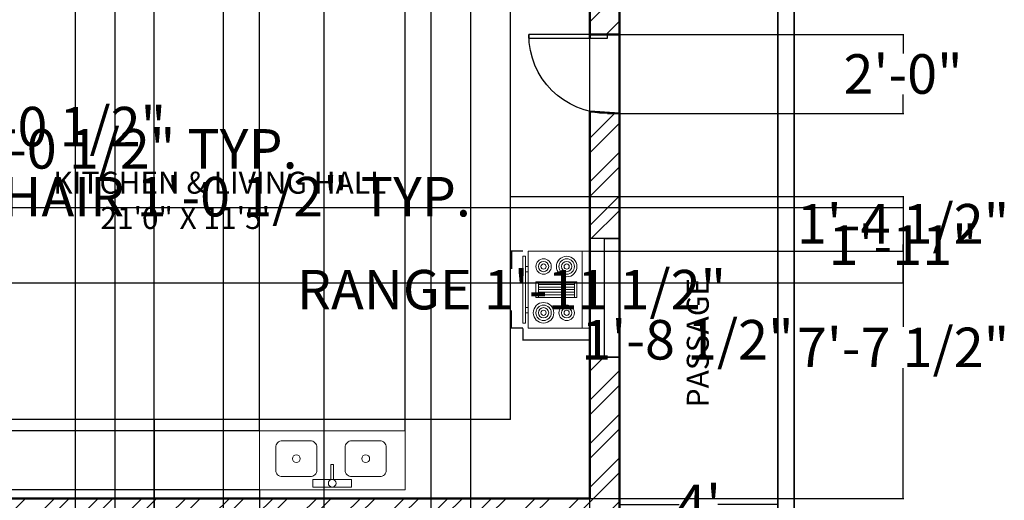
# Model space of a CAD drawing. Units: inches. Extents: x -40 to 578, y -482 to 237.
# Tile 6 of 7: x 249 to 548, y -129 to 17. Entities that reach past the tile are written whole.
import ezdxf

# ---------------------------------------------------------------- set-up
doc = ezdxf.new("R2010")
doc.units = ezdxf.units.IN
doc.header["$MEASUREMENT"] = 0
for name, color, linetype, lineweight in [('A-ANNO-DIMS', 2, 'Continuous', 18), ('A-AREA-IDEN', 240, 'Continuous', 25), ('A-EQPM', 4, 'Continuous', 18), ('A-FLOR-CASE', 4, 'Continuous', 25), ('A-FLOR-FIXT', 4, 'Continuous', 18), ('A-WALL-PATT', 252, 'Continuous', 13), ('C-PROP', 3, 'Continuous', 35), ('DOORS', 2, 'Continuous', 25), ('WALLS', 3, 'Continuous', 50), ('WINDOWS', 241, 'Continuous', 25)]:
    doc.layers.add(name, color=color, linetype=linetype, lineweight=lineweight)
doc.styles.get("Standard").update_dxf_attribs({"font": 'arial.ttf'})
doc.dimstyles.get("Standard").update_dxf_attribs({"dimtxt": 12, "dimasz": 0.18, "dimexe": 0.18, "dimexo": 0.0625, "dimgap": 0.09, "dimtad": 0, "dimtih": 1, "dimtoh": 1, "dimdec": 0, "dimzin": 0, "dimdsep": 46, "dimlunit": 3, "dimtxsty": 'Standard', "dimcen": 0.09, "dimadec": 0, "dimazin": 0, "dimtfac": 1, "dimtdec": 0, "dimtofl": 0, "dimtmove": 0, "dimatfit": 3, "dimfxl": 1, "dimtolj": 1, "dimtzin": 0, "dimarcsym": 0})

# ---------------------------------------------------------------- blocks, each defined once
blk = doc.blocks.new('Range-Oven - 30 in top')
for p, q in [((0, -3), (30, -3)), ((12, -6), (18, -6)), ((13, -20), (13, -6)), ((14, -6), (14, -20)), ((15, -20), (15, -6)), ((16, -6), (16, -20)), ((17, -20), (17, -6)), ((18, -20), (12, -20)), ((6, -24), (6, -25)), ((8, -25), (8, -24)), ((22, -25), (22, -24)), ((24, -24), (24, -25))]:
    blk.add_line(p, q)
for points in [[(0, -24), (0, 0), (30, 0), (30, -24)], [(12, -21), (12, -5), (18, -5), (18, -21)], [(2, -26), (2, -25), (28, -25), (28, -26)]]:
    blk.add_lwpolyline(points, close=True)
for centre, radius in [((6, -9), 4), ((6, -9), 3), ((6, -9), 2), ((24, -9), 3), ((24, -9), 2), ((6, -9), 1), ((24, -9), 1), ((6, -18), 3), ((24, -18), 4), ((24, -18), 3), ((6, -18), 2), ((6, -18), 1), ((24, -18), 2), ((24, -18), 1)]:
    blk.add_circle(centre, radius)
blk = doc.blocks.new('*U10')
for p, q in [((0, 0), (0, -6)), ((40, 0), (40, -6))]:
    blk.add_line(p, q)
blk.add_lwpolyline([(0, 0), (0, 40), (1.75, 40), (1.75, 0)], close=True)
blk.add_arc((0, 0), 40, 0, 90)
blk = doc.blocks.new('*D19')
at = {"layer": 'A-ANNO-DIMS', "color": 0, "lineweight": -2, "transparency": 16777216}
for p, q in [((430.74, -125.2), (430.74, -130.58)), ((478.74, -125.2), (478.74, -130.58)), ((430.92, -130.4), (448.89, -130.4)), ((478.56, -130.4), (460.59, -130.4))]:
    blk.add_line(p, q, dxfattribs=at)
at = {"layer": 'A-ANNO-DIMS', "color": 0, "transparency": 16777216}
for points in [[(430.92, -130.37), (430.92, -130.43), (430.74, -130.4)], [(478.56, -130.37), (478.56, -130.43), (478.74, -130.4)]]:
    blk.add_solid(points, dxfattribs=at)
at = {"layer": 'Defpoints', "color": 0, "transparency": 16777216}
for p in [(430.74, -125.13), (478.74, -125.13), (478.74, -130.4)]:
    blk.add_point(p, dxfattribs=at)
at = {"layer": 'A-ANNO-DIMS', "color": 0, "transparency": 16777216, "insert": (454.74, -130.4), "char_height": 12, "attachment_point": 5}
blk.add_mtext("\\A1;4'", dxfattribs=at)
blk = doc.blocks.new('WIN-36IN')
for p, q in [((9, 36), (0, 36)), ((4.5, 0), (4.5, 36)), ((4.5, 36), (9, 36)), ((9, 0), (0, 0)), ((4.5, 0), (9, 0))]:
    blk.add_line(p, q)
blk = doc.blocks.new('*D30')
at = {"layer": 'A-ANNO-DIMS', "color": 0, "lineweight": -2, "transparency": 16777216}
for p, q in [((217.52, -35.11), (217.52, -37.13)), ((230.16, -35.11), (230.16, -37.13)), ((217.7, -36.95), (229.98, -36.95)), ((230.16, -36.95), (230.34, -36.95))]:
    blk.add_line(p, q, dxfattribs=at)
at = {"layer": 'A-ANNO-DIMS', "color": 0, "transparency": 16777216}
for points in [[(217.7, -36.92), (217.7, -36.98), (217.52, -36.95)], [(229.98, -36.92), (229.98, -36.98), (230.16, -36.95)]]:
    blk.add_solid(points, dxfattribs=at)
at = {"layer": 'Defpoints', "color": 0, "transparency": 16777216}
for p in [(217.52, -35.05), (230.16, -35.05), (230.16, -36.95)]:
    blk.add_point(p, dxfattribs=at)
at = {"layer": 'A-ANNO-DIMS', "color": 0, "transparency": 16777216, "insert": (309.32, -36.95), "char_height": 12, "attachment_point": 5}
blk.add_mtext('\\A1;CHAIR 1\'-0 1/2" TYP.', dxfattribs=at)
blk = doc.blocks.new('*D31')
at = {"layer": 'A-ANNO-DIMS', "color": 0, "lineweight": -2, "transparency": 16777216}
for p, q in [((230.22, -22.61), (232.23, -22.61)), ((232.05, -22.61), (232.05, -22.43)), ((232.05, -22.43), (232.23, -22.43)), ((232.05, -34.87), (232.05, -22.79)), ((230.22, -35.05), (232.23, -35.05))]:
    blk.add_line(p, q, dxfattribs=at)
at = {"layer": 'A-ANNO-DIMS', "color": 0, "transparency": 16777216}
for points in [[(232.02, -22.79), (232.08, -22.79), (232.05, -22.61)], [(232.02, -34.87), (232.08, -34.87), (232.05, -35.05)]]:
    blk.add_solid(points, dxfattribs=at)
at = {"layer": 'Defpoints', "color": 0, "transparency": 16777216}
for p in [(230.16, -22.61), (232.05, -22.61), (230.16, -35.05)]:
    blk.add_point(p, dxfattribs=at)
at = {"layer": 'A-ANNO-DIMS', "color": 0, "transparency": 16777216, "insert": (282.31, -22.43), "char_height": 12, "attachment_point": 5}
blk.add_mtext('\\A1;1\'-0 1/2" TYP.', dxfattribs=at)
blk = doc.blocks.new('*D40')
at = {"layer": 'A-ANNO-DIMS', "color": 0, "lineweight": -2, "transparency": 16777216}
for p, q in [((401.4, -53.48), (397.77, -53.48)), ((397.95, -53.66), (397.95, -58.88)), ((397.95, -76.7), (397.95, -71.47)), ((401.4, -76.88), (397.77, -76.88))]:
    blk.add_line(p, q, dxfattribs=at)
at = {"layer": 'A-ANNO-DIMS', "color": 0, "transparency": 16777216}
for points in [[(397.92, -53.66), (397.98, -53.66), (397.95, -53.48)], [(397.92, -76.7), (397.98, -76.7), (397.95, -76.88)]]:
    blk.add_solid(points, dxfattribs=at)
at = {"layer": 'Defpoints', "color": 0, "transparency": 16777216}
for p in [(401.46, -53.48), (397.95, -76.88), (401.46, -76.88)]:
    blk.add_point(p, dxfattribs=at)
at = {"layer": 'A-ANNO-DIMS', "color": 0, "transparency": 16777216, "insert": (397.95, -65.18), "char_height": 12, "attachment_point": 5}
blk.add_mtext('\\A1;RANGE 1\'-11 1/2"', dxfattribs=at)
blk = doc.blocks.new('*D41')
at = {"layer": 'A-ANNO-DIMS', "color": 0, "lineweight": -2, "transparency": 16777216}
for p, q in [((401.46, -76.94), (401.46, -80.57)), ((421.74, -76.94), (421.74, -80.57)), ((401.64, -80.39), (421.56, -80.39)), ((421.74, -80.39), (421.92, -80.39))]:
    blk.add_line(p, q, dxfattribs=at)
at = {"layer": 'A-ANNO-DIMS', "color": 0, "transparency": 16777216}
for points in [[(401.64, -80.36), (401.64, -80.42), (401.46, -80.39)], [(421.56, -80.36), (421.56, -80.42), (421.74, -80.39)]]:
    blk.add_solid(points, dxfattribs=at)
at = {"layer": 'Defpoints', "color": 0, "transparency": 16777216}
for p in [(401.46, -76.88), (421.74, -76.88), (421.74, -80.39)]:
    blk.add_point(p, dxfattribs=at)
at = {"layer": 'A-ANNO-DIMS', "color": 0, "transparency": 16777216, "insert": (451.37, -80.39), "char_height": 12, "attachment_point": 5}
blk.add_mtext('\\A1;1\'-8 1/2"', dxfattribs=at)
blk = doc.blocks.new('*D49')
at = {"layer": 'A-ANNO-DIMS', "color": 0, "lineweight": -2, "transparency": 16777216}
for p, q in [((385.66, -377.49), (385.66, 219.12)), ((385.84, 218.94), (387.66, 218.94)), ((421.56, 218.94), (419.73, 218.94)), ((421.74, -377.49), (421.74, 219.12))]:
    blk.add_line(p, q, dxfattribs=at)
at = {"layer": 'A-ANNO-DIMS', "color": 0, "transparency": 16777216}
for points in [[(385.84, 218.97), (385.84, 218.91), (385.66, 218.94)], [(421.56, 218.97), (421.56, 218.91), (421.74, 218.94)]]:
    blk.add_solid(points, dxfattribs=at)
at = {"layer": 'Defpoints', "color": 0, "transparency": 16777216}
for p in [(421.74, 218.94), (385.66, -377.55), (421.74, -377.55)]:
    blk.add_point(p, dxfattribs=at)
at = {"layer": 'A-ANNO-DIMS', "color": 0, "transparency": 16777216, "insert": (403.7, 218.94), "char_height": 12, "attachment_point": 5}
blk.add_mtext('\\A1;3\'-0"', dxfattribs=at)
blk = doc.blocks.new('*D50')
at = {"layer": 'A-ANNO-DIMS', "color": 0, "lineweight": -2, "transparency": 16777216}
for p, q in [((265.66, -330.99), (265.66, 219.12)), ((265.84, 218.94), (277.48, 218.94)), ((277.66, -330.99), (277.66, 219.12)), ((277.66, 218.94), (277.84, 218.94))]:
    blk.add_line(p, q, dxfattribs=at)
at = {"layer": 'A-ANNO-DIMS', "color": 0, "transparency": 16777216}
for points in [[(265.84, 218.97), (265.84, 218.91), (265.66, 218.94)], [(277.48, 218.97), (277.48, 218.91), (277.66, 218.94)]]:
    blk.add_solid(points, dxfattribs=at)
at = {"layer": 'Defpoints', "color": 0, "transparency": 16777216}
for p in [(277.66, 218.94), (265.66, -331.05), (277.66, -331.05)]:
    blk.add_point(p, dxfattribs=at)
at = {"layer": 'A-ANNO-DIMS', "color": 0, "transparency": 16777216, "insert": (293.31, 218.94), "char_height": 12, "attachment_point": 5}
blk.add_mtext('\\A1;1\'-0"', dxfattribs=at)
blk = doc.blocks.new('*D52')
at = {"layer": 'A-ANNO-DIMS', "color": 0, "lineweight": -2, "transparency": 16777216}
for p, q in [((234.57, -377.49), (234.57, 219.12)), ((234.75, 218.94), (265.48, 218.94)), ((265.66, -377.49), (265.66, 219.12)), ((265.66, 218.94), (265.84, 218.94))]:
    blk.add_line(p, q, dxfattribs=at)
at = {"layer": 'A-ANNO-DIMS', "color": 0, "transparency": 16777216}
for points in [[(234.75, 218.97), (234.75, 218.91), (234.57, 218.94)], [(265.48, 218.97), (265.48, 218.91), (265.66, 218.94)]]:
    blk.add_solid(points, dxfattribs=at)
at = {"layer": 'Defpoints', "color": 0, "transparency": 16777216}
for p in [(265.66, 218.94), (234.57, -377.55), (265.66, -377.55)]:
    blk.add_point(p, dxfattribs=at)
at = {"layer": 'A-ANNO-DIMS', "color": 0, "transparency": 16777216, "insert": (281.98, 218.94), "char_height": 12, "attachment_point": 5}
blk.add_mtext('\\A1;2\'-7"', dxfattribs=at)
blk = doc.blocks.new('*D59')
at = {"layer": 'A-ANNO-DIMS', "color": 0, "lineweight": -2, "transparency": 16777216}
for p, q in [((430.8, 12.26), (516.97, 12.26)), ((516.79, 12.08), (516.79, 6.51)), ((516.79, -11.49), (516.79, -5.92)), ((430.8, -11.67), (516.97, -11.67))]:
    blk.add_line(p, q, dxfattribs=at)
at = {"layer": 'A-ANNO-DIMS', "color": 0, "transparency": 16777216}
for points in [[(516.76, 12.08), (516.82, 12.08), (516.79, 12.26)], [(516.76, -11.49), (516.82, -11.49), (516.79, -11.67)]]:
    blk.add_solid(points, dxfattribs=at)
at = {"layer": 'Defpoints', "color": 0, "transparency": 16777216}
for p in [(430.74, 12.26), (516.79, 12.26), (430.74, -11.67)]:
    blk.add_point(p, dxfattribs=at)
at = {"layer": 'A-ANNO-DIMS', "color": 0, "transparency": 16777216, "insert": (516.79, 0.3), "char_height": 12, "attachment_point": 5}
blk.add_mtext('\\A1;2\'-0"', dxfattribs=at)
blk = doc.blocks.new('*D63')
at = {"layer": 'A-ANNO-DIMS', "color": 0, "lineweight": -2, "transparency": 16777216}
for p, q in [((289.56, -104.49), (289.56, 219.12)), ((289.74, 218.94), (327.56, 218.94)), ((397.45, 218.94), (359.64, 218.94)), ((397.63, -104.49), (397.63, 219.12))]:
    blk.add_line(p, q, dxfattribs=at)
at = {"layer": 'A-ANNO-DIMS', "color": 0, "transparency": 16777216}
for points in [[(289.74, 218.97), (289.74, 218.91), (289.56, 218.94)], [(397.45, 218.97), (397.45, 218.91), (397.63, 218.94)]]:
    blk.add_solid(points, dxfattribs=at)
at = {"layer": 'Defpoints', "color": 0, "transparency": 16777216}
for p in [(397.63, 218.94), (289.56, -104.55), (397.63, -104.55)]:
    blk.add_point(p, dxfattribs=at)
at = {"layer": 'A-ANNO-DIMS', "color": 0, "transparency": 16777216, "insert": (343.6, 218.94), "char_height": 12, "attachment_point": 5}
blk.add_mtext('\\A1;9\'-0"', dxfattribs=at)
blk = doc.blocks.new('*D64')
at = {"layer": 'A-ANNO-DIMS', "color": 0, "lineweight": -2, "transparency": 16777216}
for p, q in [((397.63, -36.81), (397.63, 219.12)), ((397.81, 218.94), (421.56, 218.94)), ((421.74, -36.81), (421.74, 219.12)), ((421.74, 218.94), (421.92, 218.94))]:
    blk.add_line(p, q, dxfattribs=at)
at = {"layer": 'A-ANNO-DIMS', "color": 0, "transparency": 16777216}
for points in [[(397.81, 218.97), (397.81, 218.91), (397.63, 218.94)], [(421.56, 218.97), (421.56, 218.91), (421.74, 218.94)]]:
    blk.add_solid(points, dxfattribs=at)
at = {"layer": 'Defpoints', "color": 0, "transparency": 16777216}
for p in [(421.74, 218.94), (397.63, -36.87), (421.74, -36.87)]:
    blk.add_point(p, dxfattribs=at)
at = {"layer": 'A-ANNO-DIMS', "color": 0, "transparency": 16777216, "insert": (438.06, 218.94), "char_height": 12, "attachment_point": 5}
blk.add_mtext('\\A1;2\'-0"', dxfattribs=at)
blk = doc.blocks.new('*D65')
at = {"layer": 'A-ANNO-DIMS', "color": 0, "lineweight": -2, "transparency": 16777216}
for p, q in [((421.8, -36.87), (516.97, -36.87)), ((516.79, -37.05), (516.79, -76.42)), ((516.79, -128.37), (516.79, -89)), ((421.8, -128.55), (516.97, -128.55))]:
    blk.add_line(p, q, dxfattribs=at)
at = {"layer": 'A-ANNO-DIMS', "color": 0, "transparency": 16777216}
for points in [[(516.76, -37.05), (516.82, -37.05), (516.79, -36.87)], [(516.76, -128.37), (516.82, -128.37), (516.79, -128.55)]]:
    blk.add_solid(points, dxfattribs=at)
at = {"layer": 'Defpoints', "color": 0, "transparency": 16777216}
for p in [(421.74, -36.87), (421.74, -128.55), (516.79, -128.55)]:
    blk.add_point(p, dxfattribs=at)
at = {"layer": 'A-ANNO-DIMS', "color": 0, "transparency": 16777216, "insert": (516.79, -82.71), "char_height": 12, "attachment_point": 5}
blk.add_mtext('\\A1;7\'-7 1/2"', dxfattribs=at)
blk = doc.blocks.new('*D66')
at = {"layer": 'A-ANNO-DIMS', "color": 0, "lineweight": -2, "transparency": 16777216}
for p, q in [((289.5, -104.55), (-3.49, -104.55)), ((-3.31, -104.73), (-3.31, -110.34)), ((-3.31, -128.37), (-3.31, -122.77)), ((289.5, -128.55), (-3.49, -128.55))]:
    blk.add_line(p, q, dxfattribs=at)
at = {"layer": 'A-ANNO-DIMS', "color": 0, "transparency": 16777216}
for points in [[(-3.34, -104.73), (-3.28, -104.73), (-3.31, -104.55)], [(-3.34, -128.37), (-3.28, -128.37), (-3.31, -128.55)]]:
    blk.add_solid(points, dxfattribs=at)
at = {"layer": 'Defpoints', "color": 0, "transparency": 16777216}
for p in [(289.56, -104.55), (-3.31, -128.55), (289.56, -128.55)]:
    blk.add_point(p, dxfattribs=at)
at = {"layer": 'A-ANNO-DIMS', "color": 0, "transparency": 16777216, "insert": (-3.31, -116.55), "char_height": 12, "attachment_point": 5}
blk.add_mtext('\\A1;2\'-0"', dxfattribs=at)
blk = doc.blocks.new('*D67')
at = {"layer": 'A-ANNO-DIMS', "color": 0, "lineweight": -2, "transparency": 16777216}
for p, q in [((321.5, -108), (321.5, 219.12)), ((321.68, 218.94), (327.57, 218.94)), ((365.53, 218.94), (359.64, 218.94)), ((365.71, -108), (365.71, 219.12))]:
    blk.add_line(p, q, dxfattribs=at)
at = {"layer": 'A-ANNO-DIMS', "color": 0, "transparency": 16777216}
for points in [[(321.68, 218.97), (321.68, 218.91), (321.5, 218.94)], [(365.53, 218.97), (365.53, 218.91), (365.71, 218.94)]]:
    blk.add_solid(points, dxfattribs=at)
at = {"layer": 'Defpoints', "color": 0, "transparency": 16777216}
for p in [(365.71, 218.94), (321.5, -108.06), (365.71, -108.06)]:
    blk.add_point(p, dxfattribs=at)
at = {"layer": 'A-ANNO-DIMS', "color": 0, "transparency": 16777216, "insert": (343.6, 218.94), "char_height": 12, "attachment_point": 5}
blk.add_mtext('\\A1;3\'-8"', dxfattribs=at)
blk = doc.blocks.new('*D68')
at = {"layer": 'A-ANNO-DIMS', "color": 0, "lineweight": -2, "transparency": 16777216}
for p, q in [((321.44, -108.06), (-3.49, -108.06)), ((-3.31, -108.24), (-3.31, -110.78)), ((-3.31, -125.74), (-3.31, -123.21)), ((321.44, -125.92), (-3.49, -125.92))]:
    blk.add_line(p, q, dxfattribs=at)
at = {"layer": 'A-ANNO-DIMS', "color": 0, "transparency": 16777216}
for points in [[(-3.34, -108.24), (-3.28, -108.24), (-3.31, -108.06)], [(-3.34, -125.74), (-3.28, -125.74), (-3.31, -125.92)]]:
    blk.add_solid(points, dxfattribs=at)
at = {"layer": 'Defpoints', "color": 0, "transparency": 16777216}
for p in [(321.5, -108.06), (-3.31, -125.92), (321.5, -125.92)]:
    blk.add_point(p, dxfattribs=at)
at = {"layer": 'A-ANNO-DIMS', "color": 0, "transparency": 16777216, "insert": (-3.31, -116.99), "char_height": 12, "attachment_point": 5}
blk.add_mtext('\\A1;1\'-6"', dxfattribs=at)
blk = doc.blocks.new('*D69')
at = {"layer": 'A-ANNO-DIMS', "color": 0, "lineweight": -2, "transparency": 16777216}
for p, q in [((321.5, -125.98), (321.5, -474.78)), ((289.56, -128.61), (289.56, -474.78)), ((289.74, -474.6), (321.32, -474.6)), ((321.5, -474.6), (321.68, -474.6))]:
    blk.add_line(p, q, dxfattribs=at)
at = {"layer": 'A-ANNO-DIMS', "color": 0, "transparency": 16777216}
for points in [[(289.74, -474.57), (289.74, -474.63), (289.56, -474.6)], [(321.32, -474.57), (321.32, -474.63), (321.5, -474.6)]]:
    blk.add_solid(points, dxfattribs=at)
at = {"layer": 'Defpoints', "color": 0, "transparency": 16777216}
for p in [(321.5, -125.92), (289.56, -128.55), (321.5, -474.6)]:
    blk.add_point(p, dxfattribs=at)
at = {"layer": 'A-ANNO-DIMS', "color": 0, "transparency": 16777216, "insert": (337.82, -474.6), "char_height": 12, "attachment_point": 5}
blk.add_mtext('\\A1;2\'-8"', dxfattribs=at)
blk = doc.blocks.new('*D72')
at = {"layer": 'A-ANNO-DIMS', "color": 0, "lineweight": -2, "transparency": 16777216}
for p, q in [((238.04, -40.21), (516.97, -40.21)), ((516.79, -40.39), (516.79, -45.55)), ((516.79, -62.94), (516.79, -57.78)), ((238.04, -63.12), (516.97, -63.12))]:
    blk.add_line(p, q, dxfattribs=at)
at = {"layer": 'A-ANNO-DIMS', "color": 0, "transparency": 16777216}
for points in [[(516.76, -40.39), (516.82, -40.39), (516.79, -40.21)], [(516.76, -62.94), (516.82, -62.94), (516.79, -63.12)]]:
    blk.add_solid(points, dxfattribs=at)
at = {"layer": 'Defpoints', "color": 0, "transparency": 16777216}
for p in [(237.97, -40.21), (516.79, -40.21), (237.97, -63.12)]:
    blk.add_point(p, dxfattribs=at)
at = {"layer": 'A-ANNO-DIMS', "color": 0, "transparency": 16777216, "insert": (516.79, -51.67), "char_height": 12, "attachment_point": 5}
blk.add_mtext('\\A1;1\'-11"', dxfattribs=at)
blk = doc.blocks.new('*D73')
at = {"layer": 'A-ANNO-DIMS', "color": 0, "lineweight": -2, "transparency": 16777216}
for p, q in [((289.59, -268.55), (289.59, 219.12)), ((289.77, 218.94), (315.6, 218.94)), ((373.41, 218.94), (347.58, 218.94)), ((373.59, -268.55), (373.59, 219.12))]:
    blk.add_line(p, q, dxfattribs=at)
at = {"layer": 'A-ANNO-DIMS', "color": 0, "transparency": 16777216}
for points in [[(289.77, 218.97), (289.77, 218.91), (289.59, 218.94)], [(373.41, 218.97), (373.41, 218.91), (373.59, 218.94)]]:
    blk.add_solid(points, dxfattribs=at)
at = {"layer": 'Defpoints', "color": 0, "transparency": 16777216}
for p in [(373.59, 218.94), (289.59, -268.61), (373.59, -268.61)]:
    blk.add_point(p, dxfattribs=at)
at = {"layer": 'A-ANNO-DIMS', "color": 0, "transparency": 16777216, "insert": (331.59, 218.94), "char_height": 12, "attachment_point": 5}
blk.add_mtext('\\A1;7\'-0"', dxfattribs=at)
blk = doc.blocks.new('*D75')
at = {"layer": 'A-ANNO-DIMS', "color": 0, "lineweight": -2, "transparency": 16777216}
for p, q in [((310.54, -218.11), (310.54, 219.12)), ((310.72, 218.94), (340.99, 218.94)), ((341.17, -218.11), (341.17, 219.12)), ((341.17, 218.94), (341.35, 218.94))]:
    blk.add_line(p, q, dxfattribs=at)
at = {"layer": 'A-ANNO-DIMS', "color": 0, "transparency": 16777216}
for points in [[(310.72, 218.97), (310.72, 218.91), (310.54, 218.94)], [(340.99, 218.97), (340.99, 218.91), (341.17, 218.94)]]:
    blk.add_solid(points, dxfattribs=at)
at = {"layer": 'Defpoints', "color": 0, "transparency": 16777216}
for p in [(341.17, 218.94), (310.54, -218.17), (341.17, -218.17)]:
    blk.add_point(p, dxfattribs=at)
at = {"layer": 'A-ANNO-DIMS', "color": 0, "transparency": 16777216, "insert": (371.48, 218.94), "char_height": 12, "attachment_point": 5}
blk.add_mtext('\\A1;2\'-6 1/2"', dxfattribs=at)
blk = doc.blocks.new('*D79')
at = {"layer": 'A-ANNO-DIMS', "color": 0, "lineweight": -2, "transparency": 16777216}
for p, q in [((421.8, -36.87), (516.97, -36.87)), ((516.79, -37.05), (516.79, -38.88)), ((421.8, -53.48), (516.97, -53.48)), ((516.79, -53.3), (516.79, -51.47))]:
    blk.add_line(p, q, dxfattribs=at)
at = {"layer": 'A-ANNO-DIMS', "color": 0, "transparency": 16777216}
for points in [[(516.76, -37.05), (516.82, -37.05), (516.79, -36.87)], [(516.76, -53.3), (516.82, -53.3), (516.79, -53.48)]]:
    blk.add_solid(points, dxfattribs=at)
at = {"layer": 'Defpoints', "color": 0, "transparency": 16777216}
for p in [(421.74, -36.87), (516.79, -36.87), (421.74, -53.48)]:
    blk.add_point(p, dxfattribs=at)
at = {"layer": 'A-ANNO-DIMS', "color": 0, "transparency": 16777216, "insert": (516.79, -45.17), "char_height": 12, "attachment_point": 5}
blk.add_mtext('\\A1;1\'-4 1/2"', dxfattribs=at)
blk = doc.blocks.new('*D82')
at = {"layer": 'A-ANNO-DIMS', "color": 0, "lineweight": -2, "transparency": 16777216}
for p, q in [((196.01, -15.68), (195.83, -15.68)), ((195.83, -15.68), (195.83, -22.89)), ((195.74, -35.39), (195.92, -35.39)), ((195.83, -35.48), (195.83, -35.3))]:
    blk.add_line(p, q, dxfattribs=at)
at = {"layer": 'A-ANNO-DIMS', "color": 0, "transparency": 16777216}
blk.add_solid([(195.8, -22.89), (195.86, -22.89), (195.83, -23.07)], dxfattribs=at)
at = {"layer": 'Defpoints', "color": 0, "transparency": 16777216}
for p in [(195.83, -23.07), (195.83, -35.39)]:
    blk.add_point(p, dxfattribs=at)
at = {"layer": 'A-ANNO-DIMS', "color": 0, "transparency": 16777216, "insert": (244.7, -15.68), "char_height": 12, "attachment_point": 5}
blk.add_mtext('\\A1;6X R1\'-0 1/2"', dxfattribs=at)

msp = doc.modelspace()

# ---------------------------------------------------------------- hatches: boundary and pattern name
at = {"layer": 'A-WALL-PATT'}
h = msp.add_hatch(dxfattribs=at)
h.set_pattern_fill('ANSI32', color=256, scale=25)
h.set_pattern_definition([(45, (-1993.713, -1175.095), (-6.629126, 6.629126), []), (45, (-1989.294, -1175.095), (-6.629126, 6.629126), [])])
h.paths.add_polyline_path([(248.74, 172.45), (71.74, 172.45), (71.74, 114.63), (80.74, 114.63), (80.74, 163.45), (248.74, 163.45)])
h.paths.add_polyline_path([(253.74, 172.45), (248.74, 172.45), (248.74, 163.45), (253.74, 163.45)])
h.paths.add_polyline_path([(253.74, 163.45), (248.74, 163.45), (248.74, 25.45), (240.62, 25.45), (240.62, 20.45), (263.71, 20.45), (263.71, 25.45), (253.74, 25.45)])
h.paths.add_polyline_path([(483.74, 172.45), (253.74, 172.45), (253.74, 163.45), (426.74, 163.45), (474.74, 163.45), (474.74, 79.45), (465.23, 79.45), (465.23, 77.2), (441.23, 77.2), (441.23, 74.45), (483.74, 74.45)])
h.paths.add_polyline_path([(80.74, 78.63), (71.74, 78.63), (71.74, 3.32), (80.74, 3.32), (80.74, 20.45), (134.6, 20.45), (134.6, 25.45), (80.74, 25.45)])
h.paths.add_polyline_path([(202.4, 25.45), (158.53, 25.45), (158.53, 20.45), (202.4, 20.45)])
h.paths.add_polyline_path([(169.74, 20.45), (164.74, 20.45), (164.74, -39.55), (80.74, -39.55), (80.74, -20.68), (71.74, -20.68), (71.74, -61.38), (80.74, -61.38), (80.74, -44.55), (164.74, -44.55), (164.74, -104.55), (169.74, -104.55), (169.74, -44.55)])
h.paths.add_polyline_path([(135.96, -104.55), (80.74, -104.55), (80.74, -85.38), (71.74, -85.38), (71.74, -155.89), (80.74, -155.89), (80.74, -109.55), (135.96, -109.55)])
h.paths.add_polyline_path([(218.74, -104.55), (159.9, -104.55), (159.9, -109.55), (218.74, -109.55)])
h.paths.add_polyline_path([(223.74, -104.55), (218.74, -104.55), (218.74, -109.55), (223.74, -109.55)])
h.paths.add_polyline_path([(223.74, -109.55), (218.74, -109.55), (218.74, -114.58), (223.74, -114.58)])
h.paths.add_polyline_path([(430.74, -85.66), (421.74, -85.66), (421.74, -128.55), (223.74, -128.55), (223.74, -133.55), (421.74, -133.55), (421.74, -197.77), (430.74, -197.77)])
h.paths.add_polyline_path([(223.74, -152.8), (218.74, -152.8), (218.74, -229.55), (151.59, -229.55), (151.59, -238.55), (223.74, -238.55), (223.74, -229.55)])
h.paths.add_polyline_path([(115.59, -229.55), (98.23, -229.55), (80.74, -229.55), (80.74, -212.75), (80.74, -191.89), (71.74, -191.89), (71.74, -238.55), (115.59, -238.55)])
h.paths.add_polyline_path([(307.53, -289.55), (223.74, -289.55), (223.74, -283.47), (218.74, -283.47), (218.74, -298.55), (307.53, -298.55)])
h.paths.add_polyline_path([(421.74, -289.55), (343.53, -289.55), (343.53, -298.55), (421.74, -298.55)])
h.paths.add_polyline_path([(430.74, -367.34), (421.74, -367.34), (421.74, -377.55), (234.57, -377.55), (234.57, -386.55), (430.74, -386.55)])
h.paths.add_polyline_path([(430.74, -298.55), (430.74, -233.77), (421.74, -233.77), (421.74, -289.55), (421.74, -298.55), (421.74, -331.34), (430.74, -331.34)])
h.paths.add_polyline_path([(430.74, -11.67), (427.15, -11.67, -0.057068), (421.74, -11.05), (421.74, -49.66), (430.74, -49.66)])
h.paths.add_polyline_path([(430.74, 31.9), (421.74, 31.9), (421.74, 25.45), (301.93, 25.45), (301.93, 20.45), (421.74, 20.45), (421.74, 12.26), (430.74, 12.26)])
h.paths.add_polyline_path([(426.74, 134.23, -0.014739), (425.33, 134.19), (421.74, 134.19), (421.74, 74.45), (441.23, 74.45), (441.23, 77.2), (441.23, 79.45), (426.74, 79.45)], flags=17)
h.paths.add_polyline_path([(430.74, 74.45), (421.74, 74.45), (421.74, 67.9), (430.74, 67.9)])

# ---------------------------------------------------------------- linework, layer by layer
at = {"layer": 'A-FLOR-CASE'}
for p, q in [((397.63, -104.55), (397.63, -36.87)), ((397.63, -36.87), (421.74, -36.87)), ((397.63, -104.55), (289.56, -104.55)), ((289.56, -104.55), (289.56, -128.55))]:
    msp.add_line(p, q, dxfattribs=at)
at = {"layer": 'A-FLOR-FIXT'}
for points in [[(365.71, -125.92), (321.5, -125.92), (321.5, -108.06), (365.71, -108.06)], [(343.91, -122.78), (343.2, -122.78), (343.2, -118.28), (343.91, -118.28)], [(349.42, -125.1), (337.7, -125.1), (337.7, -122.78), (349.42, -122.78)]]:
    msp.add_lwpolyline(points, close=True, dxfattribs=at)
for points in [[(336.93, -121.95), (328.43, -121.95, -0.414214), (326.43, -119.95), (326.43, -113.05, -0.414214), (328.43, -111.05), (336.93, -111.05, -0.414214), (338.93, -113.05), (338.93, -119.95, -0.414214)], [(357.99, -121.95), (349.49, -121.95, -0.414214), (347.49, -119.95), (347.49, -113.05, -0.414214), (349.49, -111.05), (357.99, -111.05, -0.414214), (359.99, -113.05), (359.99, -119.95, -0.414214)]]:
    msp.add_lwpolyline(points, format="xyb", close=True, dxfattribs=at)
for centre, radius in [((332.68, -116.5), 1.19), ((353.74, -116.5), 1.19), ((343.56, -123.94), 1.16)]:
    msp.add_circle(centre, radius, dxfattribs=at)
at = {"layer": 'C-PROP'}
for p, q in [((478.74, 74.45), (478.74, -432.55)), ((483.74, 74.45), (483.74, -441.55))]:
    msp.add_line(p, q, dxfattribs=at)
at = {"layer": 'WALLS'}
for p, q in [((430.74, 74.45), (430.74, -298.55)), ((421.74, 20.45), (421.74, 11.22)), ((421.74, 12.26), (430.74, 12.26)), ((430.74, -11.67), (421.74, -11.05)), ((421.74, -11.05), (421.74, -128.55)), ((223.74, -128.55), (421.74, -128.55))]:
    msp.add_line(p, q, dxfattribs=at)

# ---------------------------------------------------------------- block references
at = {"layer": 'A-EQPM', "xscale": 0.7799837543148895, "yscale": 0.7799837543148895, "zscale": 0.7799837543148895, "rotation": 270}
msp.add_blockref('Range-Oven - 30 in top', (421.74, -53.48), dxfattribs=at)
at = {"layer": 'DOORS', "xscale": -0.5983195859330738, "yscale": 0.5983195859330738, "zscale": 0.5983195859330738, "rotation": 90}
msp.add_blockref('*U10', (427.15, 12.26), dxfattribs=at)
at = {"layer": 'WINDOWS'}
msp.add_blockref('WIN-36IN', (421.74, -85.66), dxfattribs=at)

# ---------------------------------------------------------------- texts
at = {"layer": 'A-AREA-IDEN'}
for s, p in [('KITCHEN & LIVING HALL', (258.94, -36.04)), ('       21\'0" X 11\'5\'', (258.94, -46.75))]:
    msp.add_text(s, height=6.6698, dxfattribs=at).set_placement(p)
msp.add_text('PASSAGE', height=6.67, rotation=90, dxfattribs=at).set_placement((457.83, -100.91))

# ---------------------------------------------------------------- dimensions: what is measured, and where the dimension line sits
at = {"layer": 'A-ANNO-DIMS'}
for base, p1, p2, override, picture, middle in [((341.17, 218.94), (310.54, -218.17), (341.17, -218.17), {"dimdec": 1, "dimlfac": 1, "dimrnd": 0, "dimzin": 1, "dimdsep": 46, "dimlunit": 4, "dimfrac": 2}, '*D75', (371.48, 218.94)), ((265.66, 218.94), (234.57, -377.55), (265.66, -377.55), {"dimdec": 1, "dimlfac": 1, "dimrnd": 0, "dimzin": 1, "dimdsep": 46, "dimlunit": 4, "dimfrac": 2}, '*D52', (281.98, 218.94)), ((277.66, 218.94), (265.66, -331.05), (277.66, -331.05), {"dimdec": 1, "dimlfac": 1, "dimrnd": 0, "dimzin": 1, "dimdsep": 46, "dimlunit": 4, "dimfrac": 2}, '*D50', (293.31, 218.94)), ((397.63, 218.94), (289.56, -104.55), (397.63, -104.55), {"dimdec": 1, "dimlfac": 1, "dimrnd": 0, "dimzin": 1, "dimdsep": 46, "dimlunit": 4, "dimfrac": 2}, '*D63', (343.6, 218.94)), ((373.59, 218.94), (289.59, -268.61), (373.59, -268.61), {"dimdec": 1, "dimlfac": 1, "dimrnd": 0, "dimzin": 1, "dimdsep": 46, "dimlunit": 4, "dimfrac": 2}, '*D73', (331.59, 218.94)), ((365.71, 218.94), (321.5, -108.06), (365.71, -108.06), {"dimdec": 1, "dimlfac": 1, "dimrnd": 0, "dimzin": 1, "dimdsep": 46, "dimlunit": 4, "dimfrac": 2}, '*D67', (343.6, 218.94)), ((421.74, 218.94), (385.66, -377.55), (421.74, -377.55), {"dimdec": 1, "dimlfac": 1, "dimrnd": 0, "dimzin": 1, "dimdsep": 46, "dimlunit": 4, "dimfrac": 2}, '*D49', (403.7, 218.94)), ((421.74, 218.94), (397.63, -36.87), (421.74, -36.87), {"dimdec": 1, "dimlfac": 1, "dimrnd": 0, "dimzin": 1, "dimdsep": 46, "dimlunit": 4, "dimfrac": 2}, '*D64', (438.06, 218.94)), ((421.74, -80.39), (401.46, -76.88), (421.74, -76.88), {"dimdec": 1, "dimlfac": 1, "dimrnd": 0, "dimzin": 1, "dimdsep": 46, "dimlunit": 4, "dimfrac": 2}, '*D41', (451.37, -80.39)), ((478.74, -130.4), (430.74, -125.13), (478.74, -125.13), {"dimclrd": 0, "dimclre": 0, "dimclrt": 0}, '*D19', (454.74, -130.4)), ((321.5, -474.6), (289.56, -128.55), (321.5, -125.92), {"dimdec": 1, "dimlfac": 1, "dimrnd": 0, "dimzin": 1, "dimdsep": 46, "dimlunit": 4, "dimfrac": 2}, '*D69', (337.82, -474.6))]:
    dim = msp.add_linear_dim(base=base, p1=p1, p2=p2, dimstyle='Standard', override=override, dxfattribs=at)
    dim.commit()
    dim.dimension.update_dxf_attribs({"geometry": picture, "text_midpoint": middle})
dim = msp.add_radius_dim(center=(195.83, -35.39), mpoint=(195.83, -23.07), text='6X <>', dimstyle='Standard', override={"dimdec": 1, "dimlfac": 1, "dimrnd": 0, "dimzin": 1, "dimdsep": 46, "dimlunit": 4, "dimfrac": 2}, dxfattribs=at)
dim.commit()
dim.dimension.update_dxf_attribs({"geometry": '*D82', "text_midpoint": (244.7, -15.68), "dimtype": 164})
for base, p1, p2, picture, middle in [((516.79, 12.26), (430.74, -11.67), (430.74, 12.26), '*D59', (516.79, 0.3)), ((516.79, -36.87), (421.74, -53.48), (421.74, -36.87), '*D79', (516.79, -45.17)), ((516.79, -128.55), (421.74, -36.87), (421.74, -128.55), '*D65', (516.79, -82.71)), ((516.79, -40.21), (237.97, -63.12), (237.97, -40.21), '*D72', (516.79, -51.67)), ((-3.31, -128.55), (289.56, -104.55), (289.56, -128.55), '*D66', (-3.31, -116.55)), ((-3.31, -125.92), (321.5, -108.06), (321.5, -125.92), '*D68', (-3.31, -116.99))]:
    dim = msp.add_linear_dim(base=base, p1=p1, p2=p2, angle=90, dimstyle='Standard', override={"dimdec": 1, "dimlfac": 1, "dimrnd": 0, "dimzin": 1, "dimdsep": 46, "dimlunit": 4, "dimfrac": 2}, dxfattribs=at)
    dim.commit()
    dim.dimension.update_dxf_attribs({"geometry": picture, "text_midpoint": middle})
for base, p1, p2, angle, text, picture, middle in [((232.05, -22.61), (230.16, -35.05), (230.16, -22.61), 90, '<> TYP.', '*D31', (282.31, -22.43)), ((397.95, -76.88), (401.46, -53.48), (401.46, -76.88), 270, 'RANGE <>', '*D40', (397.95, -65.18))]:
    dim = msp.add_linear_dim(base=base, p1=p1, p2=p2, angle=angle, text=text, dimstyle='Standard', override={"dimdec": 1, "dimlfac": 1, "dimrnd": 0, "dimzin": 1, "dimdsep": 46, "dimlunit": 4, "dimfrac": 2}, dxfattribs=at)
    dim.commit()
    dim.dimension.update_dxf_attribs({"geometry": picture, "text_midpoint": middle})
dim = msp.add_linear_dim(base=(230.16, -36.95), p1=(217.52, -35.05), p2=(230.16, -35.05), text='CHAIR <> TYP.', dimstyle='Standard', override={"dimdec": 1, "dimlfac": 1, "dimrnd": 0, "dimzin": 1, "dimdsep": 46, "dimlunit": 4, "dimfrac": 2}, dxfattribs=at)
dim.commit()
dim.dimension.update_dxf_attribs({"geometry": '*D30', "text_midpoint": (309.32, -36.95)})

doc.saveas('drawing.dxf')
